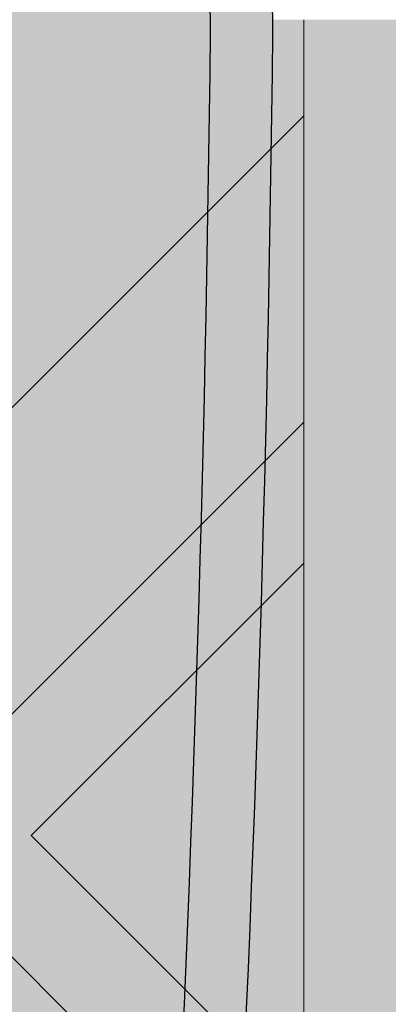
# Model space of a CAD drawing. Units: inches. Extents: x 844 to 2234, y 346 to 1084.
# Tile 11 of 93: x 1126.594 to 1127.536, y 693.702 to 696.22. Entities that reach past the tile are written whole.
import ezdxf

# ---------------------------------------------------------------- set-up
doc = ezdxf.new("R2010")
doc.units = ezdxf.units.IN
doc.header["$MEASUREMENT"] = 0
for name, color, linetype, lineweight in [('A-ANNO-DIMS', 2, 'Continuous', 18), ('furniture', 8, 'Continuous', 18), ('RA-AP-01$0$INT', 35, 'Continuous', 5)]:
    doc.layers.add(name, color=color, linetype=linetype, lineweight=lineweight)
doc.layers.add('RA-AP-01$0$FURN', color=3, linetype='Continuous')
doc.layers.add('RA-AP-01$0$WOOD', color=64, linetype='Continuous')
doc.styles.get("Standard").update_dxf_attribs({"font": 'arial.ttf'})
doc.dimstyles.get("Standard").update_dxf_attribs({"dimtxt": 6, "dimasz": 3, "dimexe": 0.18, "dimexo": 0.0625, "dimgap": 0.09, "dimtad": 0, "dimtih": 1, "dimtoh": 1, "dimdec": 1, "dimzin": 0, "dimdsep": 46, "dimlunit": 3, "dimtxsty": 'Standard', "dimblk": 'ARCHTICK', "dimcen": 0.09, "dimadec": 0, "dimazin": 0, "dimtfac": 1, "dimtdec": 1, "dimtofl": 0, "dimtmove": 0, "dimatfit": 3, "dimfxl": 1, "dimtolj": 1, "dimtzin": 0, "dimarcsym": 0})

# ---------------------------------------------------------------- blocks, each defined once
blk = doc.blocks.new('A$C18D01794')
at = {"layer": 'RA-AP-01$0$INT'}
blk.add_hatch(color=256, dxfattribs=at).paths.add_polyline_path([(4.505206456958071, -6.306712009588038), (5.305206456958072, -6.306712009588038), (5.305206456958072, -7.106712009588038), (5.255206456951893, -7.10671200958804), (5.25520645694868, -6.356712009605972), (4.555206456959269, -6.356712009587461), (4.555206456956052, -7.106712009588038), (4.505206456958073, -7.106712009588038)])
h = blk.add_hatch(color=256, dxfattribs=at)
h.paths.add_polyline_path([(4.585917135068449, -6.356712009588271), (4.555206456959269, -6.35671200958746), (4.555206456959137, -6.387422687716308), (4.874495778835233, -6.706712009592356), (4.90520645695423, -6.676001331474049)])
h.paths.add_polyline_path([(5.255206456948813, -6.387422687716306), (5.255206456948682, -6.356712009605972), (5.224495778822613, -6.356712009605161), (4.905206456953498, -6.676001331474273), (4.935917135072151, -6.706712009592924)])
h.paths.add_polyline_path([(4.935917135072559, -6.706712009592068), (4.905206456953564, -6.737422687710376), (5.255206456951813, -7.087422687708613), (5.255206456951549, -7.026001331471008)])
h.paths.add_polyline_path([(4.555206456956399, -7.026001331471013), (4.555206456956134, -7.087422687708616), (4.905206456953821, -6.737422687710943), (4.874495778835166, -6.70671200959229)])
h = blk.add_hatch(color=256, dxfattribs=at)
h.paths.add_polyline_path([(4.585917135068448, -6.356712009588273), (4.614201406330596, -6.356712009589021), (4.668846067270487, -6.411356670531338), (4.723490728212344, -6.356712009591912), (4.771774999457151, -6.35671200959319), (4.826419660396886, -6.411356670535356), (4.862780050090322, -6.374996280843536), (4.844495778842715, -6.356712009595112), (4.862780050090411, -6.356712009595595), (4.905206456960182, -6.399138416468211), (4.947632863832445, -6.356712009597838), (4.965917135079675, -6.356712009598322), (4.947632863831759, -6.374996280845421), (4.983993253523576, -6.411356670538857), (5.038637914464627, -6.356712009600247), (5.08692218571208, -6.356712009601523), (5.141566846649976, -6.411356670541852), (5.196211507589851, -6.356712009604411), (5.224495778822615, -6.356712009605161), (4.905206456953975, -6.676001331473793)])
h.paths.add_polyline_path([(4.895206456956031, -6.637717060225675), (4.895206456958921, -6.528427738347902), (4.840561796018589, -6.583072399285802)], flags=16)
h.paths.add_polyline_path([(4.915206456955638, -6.637717060226121), (4.969851117895509, -6.583072399288678), (4.915206456957609, -6.528427738348344)], flags=16)
h.paths.add_polyline_path([(4.826419660395175, -6.568930263661755), (4.881064321335613, -6.514285602723745), (4.771774999456703, -6.514285602720857)], flags=16)
h.paths.add_polyline_path([(4.983993253519558, -6.568930263665262), (5.038637914460456, -6.514285602726792), (4.929348592581548, -6.514285602724816)], flags=16)
h.paths.add_polyline_path([(4.881064321336025, -6.494285602723742), (4.826419660397532, -6.439640941782821), (4.771774999457062, -6.494285602720859)], flags=16)
h.paths.add_polyline_path([(4.929348592582019, -6.494285602724817), (5.038637914460982, -6.494285602726792), (4.983993253522945, -6.439640941786327)], flags=16)
h.paths.add_polyline_path([(4.895206456960191, -6.480143467100443), (4.895206456962115, -6.407422687715913), (4.876922185715016, -6.389138416467584), (4.840561796021581, -6.425498806159401)], flags=16)
h.paths.add_polyline_path([(4.915206456958487, -6.480143467100889), (4.969851117899527, -6.425498806162279), (4.933490728206909, -6.389138416468043), (4.9152064569598, -6.40742268771434)], flags=16)
h.paths.add_polyline_path([(4.757632863832376, -6.480143467096812), (4.812277524772842, -6.425498806158772), (4.757632863834348, -6.370854145217844)], flags=16)
h.paths.add_polyline_path([(4.737632863832376, -6.480143467096286), (4.737632863834348, -6.370854145217375), (4.682988202893906, -6.425498806155385)], flags=16)
h.paths.add_polyline_path([(5.05278005008503, -6.480143467103376), (5.052780050087917, -6.370854145224413), (4.998135389146995, -6.425498806162908)], flags=16)
h.paths.add_polyline_path([(5.072780050085024, -6.480143467103744), (5.127424711025931, -6.42549880616527), (5.072780050087916, -6.370854145224832)], flags=16)
h.paths.add_polyline_path([(4.935917135072783, -6.706712009592292), (5.255206456948811, -6.387422687716309), (5.255206456948932, -6.415706958964177), (5.200561796010279, -6.470351619902839), (5.255206456949403, -6.524996280841948), (5.25520645694961, -6.5732805520894), (5.200561796009787, -6.627925213029239), (5.236922185702417, -6.664285602721864), (5.255206456949919, -6.646001331474357), (5.255206456949998, -6.664285602721898), (5.212780050078687, -6.706712009592262), (5.25520645695036, -6.749138416463932), (5.255206456950438, -6.767422687711313), (5.236922185702424, -6.749138416463297), (5.200561796009796, -6.785498806155928), (5.255206456950753, -6.840143467096874), (5.25520645695096, -6.888427738341682), (5.200561796010322, -6.943072399282328), (5.255206456951428, -6.997717060223427), (5.255206456951547, -7.026001331471006)])
h.paths.add_polyline_path([(5.042988202883395, -6.785498806155427), (5.097632863823085, -6.840143467095101), (5.097632863822622, -6.730854145216193)], flags=16)
h.paths.add_polyline_path([(5.028846067259663, -6.771356670531693), (5.083490728198774, -6.716712009592573), (4.974201406321001, -6.716712009593042)], flags=16)
h.paths.add_polyline_path([(5.117632863823087, -6.840143467095186), (5.172277524762331, -6.785498806155926), (5.11763286382262, -6.730854145216225)], flags=16)
h.paths.add_polyline_path([(5.08349072819877, -6.696712009593886), (5.028846067259652, -6.642067348654775), (4.974201406320998, -6.696712009593438)], flags=16)
h.paths.add_polyline_path([(5.131774999446817, -6.854285602718917), (5.186419660386065, -6.799640941779662), (5.241064321325782, -6.854285602719365)], flags=17)
h.paths.add_polyline_path([(5.131774999446228, -6.716712009592374), (5.186419660386065, -6.771356670532194), (5.222780050079488, -6.734996280838764), (5.204495778832781, -6.716712009592063)], flags=16)
h.paths.add_polyline_path([(5.097632863822613, -6.682569873970264), (5.097632863823061, -6.573280552091354), (5.042988202883383, -6.627925213031044)], flags=16)
h.paths.add_polyline_path([(5.131774999446899, -6.874285602718915), (5.241064321325809, -6.874285602719364), (5.186419660386591, -6.928930263658598)], flags=17)
h.paths.add_polyline_path([(5.131774999446226, -6.696712009594078), (5.204495778830767, -6.696712009594374), (5.22278005007868, -6.67842773834687), (5.186419660386049, -6.642067348654249)], flags=16)
h.paths.add_polyline_path([(5.11763286382262, -6.682569873970225), (5.17227752476232, -6.627925213030515), (5.117632863823064, -6.573280552091267)], flags=16)
h.paths.add_polyline_path([(5.186419660386069, -6.613783077405491), (5.241064321325754, -6.559138416465795), (5.131774999446791, -6.559138416466263)], flags=16)
h.paths.add_polyline_path([(5.131774999446872, -6.539138416466263), (5.24106432132578, -6.539138416465794), (5.186419660386554, -6.484493755526573)], flags=16)
h.paths.add_polyline_path([(5.255206456951811, -7.08742268770861), (5.255206456951895, -7.106712009588038), (4.555206456956052, -7.106712009588038), (4.555206456956136, -7.087422687708617), (4.905206456953973, -6.737422687710788)])
h.paths.add_polyline_path([(4.983993253513404, -6.8444937555241), (4.92934859257295, -6.899138416462108), (5.03863791445186, -6.899138416465014)], flags=16)
h.paths.add_polyline_path([(4.969851117889988, -6.83035161990006), (4.915206456952556, -6.775706958960171), (4.915206456949648, -6.884996280837944)], flags=16)
h.paths.add_polyline_path([(4.929348592572535, -6.919138416462105), (4.983993253511019, -6.973783077403037), (5.038637914451496, -6.919138416465012)], flags=16)
h.paths.add_polyline_path([(5.052780050074912, -6.93328055208906), (4.998135389134438, -6.987925213027088), (5.052780050072919, -7.042569873968025)], flags=16)
h.paths.add_polyline_path([(5.07278005007491, -6.933280552089588), (5.072780050072918, -7.042569873968497), (5.127424711013374, -6.987925213030498)], flags=16)
h.paths.add_polyline_path([(4.89520645695295, -6.775706958959721), (4.840561796013067, -6.830351619897157), (4.895206456950961, -6.884996280837494)], flags=16)
h.paths.add_polyline_path([(4.915206456948365, -6.933280552085403), (4.915206456946434, -7.006001331471951), (4.933490728192729, -7.024285602719066), (4.969851117886972, -6.987925213026453)], flags=16)
h.paths.add_polyline_path([(4.881064321327021, -6.899138416461022), (4.82641966038902, -6.84449375552057), (4.771774999448108, -6.899138416459029)], flags=16)
h.paths.add_polyline_path([(4.895206456950073, -6.933280552084951), (4.840561796009022, -6.987925213023558), (4.876922185700835, -7.024285602716997), (4.895206456948749, -7.006001331469487)], flags=16)
h.paths.add_polyline_path([(4.983993253510392, -7.0020673486505), (4.947632863816944, -7.038427738342319), (4.965917135064043, -7.05671200959023), (5.038637914448995, -7.056712009591555)], flags=16)
h.paths.add_polyline_path([(4.881064321326543, -6.91913841646102), (4.771774999447578, -6.919138416459031), (4.826419660385607, -6.973783077399508)], flags=16)
h.paths.add_polyline_path([(4.905206456946447, -7.014285602717636), (4.862780050074785, -7.056712009588352), (4.947632863816685, -7.056712009589775)], flags=16)
h.paths.add_polyline_path([(5.14156684663679, -7.002067348654549), (5.086922185696452, -7.056712009592438), (5.196211507574223, -7.056712009594425)], flags=16)
h.paths.add_polyline_path([(4.8264196603837, -7.002067348646972), (4.771774999442643, -7.056712009585575), (4.8444957788276, -7.056712009587508), (4.862780050075511, -7.038427738340416)], flags=16)
h.paths.add_polyline_path([(4.812277524760289, -6.98792521302292), (4.757632863822258, -6.933280552082447), (4.757632863819352, -7.042569873961408)], flags=16)
h.paths.add_polyline_path([(4.73763286382226, -6.933280552082079), (4.682988202881349, -6.987925213020536), (4.737632863819352, -7.04256987396099)], flags=16)
h.paths.add_polyline_path([(4.723490728195188, -7.056712009584289), (4.668846067257299, -7.002067348643949), (4.614201406317417, -7.056712009581383)], flags=16)
h.paths.add_polyline_path([(4.597632863829262, -6.706712009592262), (4.555206456957951, -6.664285602721896), (4.555206456958029, -6.646001331474357), (4.573490728205535, -6.664285602721864), (4.609851117898167, -6.627925213029238), (4.555206456958338, -6.573280552089402), (4.555206456958546, -6.524996280841952), (4.60985111789767, -6.470351619902839), (4.555206456959015, -6.415706958964177), (4.555206456959138, -6.387422687716309), (4.874495778835167, -6.70671200959229), (4.5552064569564, -7.026001331471015), (4.555206456956523, -6.997717060223433), (4.609851117897629, -6.94307239928233), (4.555206456956988, -6.888427738341681), (4.555206456957198, -6.840143467096881), (4.609851117898153, -6.78549880615593), (4.573490728205528, -6.749138416463297), (4.555206456957507, -6.76742268771132), (4.555206456957585, -6.749138416463933)])
h.paths.add_polyline_path([(4.712780050085332, -6.730854145216195), (4.712780050084863, -6.840143467095105), (4.767424711024555, -6.785498806155427)], flags=16)
h.paths.add_polyline_path([(4.726922185709173, -6.716712009592573), (4.781566846648288, -6.771356670531693), (4.836211507586949, -6.716712009593043)], flags=16)
h.paths.add_polyline_path([(4.692780050085327, -6.730854145216225), (4.638135389145619, -6.785498806155928), (4.692780050084865, -6.840143467095185)], flags=16)
h.paths.add_polyline_path([(4.726922185709182, -6.696712009593886), (4.836211507586949, -6.696712009593436), (4.7815668466483, -6.642067348654773)], flags=16)
h.paths.add_polyline_path([(4.678637914461726, -6.71671200959237), (4.605917135075169, -6.716712009592063), (4.587632863828464, -6.734996280838766), (4.623993253521887, -6.771356670532195)], flags=16)
h.paths.add_polyline_path([(4.712780050085336, -6.68256987397026), (4.767424711024568, -6.627925213031042), (4.71278005008489, -6.573280552091352)], flags=16)
h.paths.add_polyline_path([(4.678637914461726, -6.696712009594076), (4.623993253521899, -6.642067348654247), (4.587632863829271, -6.67842773834687), (4.605917135077185, -6.696712009594376)], flags=16)
h.paths.add_polyline_path([(4.692780050085336, -6.682569873970228), (4.692780050084889, -6.573280552091267), (4.638135389145632, -6.627925213030515)], flags=16)
h.paths.add_polyline_path([(4.623993253521885, -6.799640941779662), (4.678637914461131, -6.854285602718915), (4.56934859258217, -6.854285602719365)], flags=17)
h.paths.add_polyline_path([(4.623993253521901, -6.613783077405509), (4.678637914461158, -6.559138416466263), (4.569348592582195, -6.559138416465795)], flags=16)
h.paths.add_polyline_path([(4.678637914461051, -6.874285602718915), (4.623993253521361, -6.928930263658598), (4.569348592582143, -6.874285602719364)], flags=17)
h.paths.add_polyline_path([(4.678637914461076, -6.539138416466263), (4.623993253521399, -6.484493755526573), (4.569348592582167, -6.539138416465796)], flags=16)
h = blk.add_hatch(color=256, dxfattribs=at)
h.paths.add_polyline_path([(5.028846067259997, -6.642067348655121), (4.974201406321342, -6.696712009593783), (5.083490728199115, -6.69671200959423)])
h.paths.add_polyline_path([(4.974201406321344, -6.716712009593388), (5.028846067260004, -6.771356670532039), (5.083490728199117, -6.716712009592919)])
h.paths.add_polyline_path([(5.042988202883738, -6.785498806155768), (5.097632863823428, -6.840143467095449), (5.097632863822963, -6.73085414521654)])
h.paths.add_polyline_path([(5.117632863822961, -6.730854145216568), (5.117632863823428, -6.840143467095531), (5.172277524762674, -6.785498806156272)])
h.paths.add_polyline_path([(5.131774999446572, -6.716712009592718), (5.186419660386406, -6.77135667053254), (5.222780050079831, -6.734996280839116), (5.204495778833122, -6.716712009592409)])
h.paths.add_polyline_path([(5.236922185702764, -6.749138416463644), (5.200561796010139, -6.785498806156274), (5.255206456949971, -6.840143467096101), (5.255206456950271, -6.76742268771115)])
h.paths.add_polyline_path([(5.186419660386412, -6.799640941780006), (5.131774999447164, -6.854285602719262), (5.241064321326123, -6.854285602719711)])
h.paths.add_polyline_path([(5.131774999447238, -6.874285602719261), (5.186419660386934, -6.928930263658944), (5.241064321326153, -6.874285602719709)])
h.paths.add_polyline_path([(5.200561796010663, -6.943072399282675), (5.255206456949324, -6.997717060221329), (5.255206456949777, -6.888427738343558)])
h.paths.add_polyline_path([(5.21278005007903, -6.706712009592607), (5.255206456950223, -6.749138416463798), (5.255206456950696, -6.664285602721891)])
h.paths.add_polyline_path([(5.13177499944657, -6.696712009594424), (5.204495778831106, -6.696712009594723), (5.222780050079024, -6.678427738347219), (5.186419660386397, -6.642067348654592)])
h.paths.add_polyline_path([(5.117632863823405, -6.573280552091611), (5.117632863822955, -6.682569873970578), (5.172277524762665, -6.627925213030859)])
h.paths.add_polyline_path([(5.042988202883727, -6.627925213031387), (5.097632863822957, -6.682569873970603), (5.097632863823407, -6.573280552091697)])
h.paths.add_polyline_path([(5.131774999447135, -6.559138416466609), (5.186419660386394, -6.613783077405857), (5.241064321326097, -6.559138416466144)])
h.paths.add_polyline_path([(5.200561796010128, -6.627925213029584), (5.236922185702758, -6.664285602722211), (5.255206456950264, -6.646001331474705), (5.255206456949948, -6.573280552089752)])
h.paths.add_polyline_path([(5.186419660386895, -6.484493755526919), (5.131774999447213, -6.539138416466609), (5.241064321326127, -6.539138416466142)])
h.paths.add_polyline_path([(5.200561796010624, -6.470351619903183), (5.255206456949745, -6.524996280842298), (5.255206456949276, -6.415706958964523)])
for p, q in [((5.255206456951895, -7.106712009588038), (5.255206456948681, -6.356712009605972)), ((4.935917135072783, -6.706712009592292), (5.255206456951548, -7.026001331471007)), ((4.905206456953975, -6.737422687710788), (5.255206456951811, -7.087422687708611)), ((5.241064321325809, -6.874285602719364), (5.186419660386589, -6.928930263658598)), ((5.255206456949429, -6.888427738343214), (5.200561796010322, -6.943072399282328)), ((5.255206456949433, -6.888427738343212), (5.255206456948982, -6.997717060220983)), ((5.255206456948982, -6.997717060220983), (5.200561796010322, -6.943072399282328))]:
    blk.add_line(p, q, dxfattribs=at)
blk = doc.blocks.new('A$C32926AE1')
at = {"layer": 'RA-AP-01$0$WOOD'}
h = blk.add_hatch(color=256, dxfattribs=at)
h.dxf.hatch_style = 1
h.paths.add_polyline_path([(5.157430609644524, 4.573483066760929, -0.1009492694046607), (5.155401577623758, 4.593365984175333, -0.1842662638101597), (5.172249623284174, 4.638795604568598, 0.2056608120311276), (5.179560981299304, 4.661316324430096, 0.3614336704623542), (5.134352340494423, 4.706524965234944, 0.2056608120311297), (5.111831620632933, 4.699213607219793, -0.1842662638101113), (5.066402000239693, 4.682365561559342, -0.1055311479399994), (5.045656153913092, 4.68467289944697, 0.1567636581983829), (4.763886414745334, 4.684672899446966, -0.1055311479399895), (4.743140568418733, 4.68236556155934, -0.1842662638100833), (4.6977109480255, 4.69921360721979, 0.2056608120302612), (4.675190228164109, 4.706524965234949, 0.3614336704708441), (4.629981587358889, 4.66131632442871, 0.2056608120245944), (4.637292945374126, 4.638795604567974, -0.1842662638101024), (4.654140991034615, 4.59336598417475, -0.1009492694055169), (4.652111959013835, 4.573483066760181, 0.021410119221476), (4.629748025606143, 4.156712009541676, 0.0214101192214795), (4.652111959013809, 3.739940952323101, -0.1009492694059586), (4.654140991034615, 3.720058034908448, -0.1842662638100975), (4.637292945374126, 3.674628414515226, 0.2056608120245705), (4.629981587358889, 3.652107694654492, 0.3614336704708879), (4.675190228164113, 3.606899053848249, 0.2056608120302384), (4.697710948025501, 3.614210411863408, -0.1842662638100995), (4.743140568418738, 3.63105845752386, -0.1055311479402541), (4.763886414745388, 3.628751119636215, 0.1567636581983776), (5.045656153913137, 3.628751119636244, -0.1055311479397538), (5.066402000239692, 3.631058457523857, -0.1842662638101067), (5.111831620632931, 3.614210411863407, 0.2056608120310924), (5.134352340494417, 3.606899053848256, 0.3614336704624001), (5.179560981299307, 3.652107694653103, 0.2056608120311314), (5.172249623284175, 3.6746284145146, -0.1842662638101402), (5.155401577623758, 3.72005803490786, -0.1009492694051366), (5.15743060964455, 3.739940952322354, 0.0214101192215073), (5.179794543052287, 4.156712009541468, 0.0214101192215252)])
h.paths.add_polyline_path([(4.639748609479751, 4.156712009541513, 0.0213537860821624), (4.661970494867118, 3.741887061152232, -0.094075836301374), (4.664143710413708, 3.7196126951003, -0.1824818158568985), (4.644813765429836, 3.668037719127816, 0.2056608120245319), (4.639939526753007, 3.653023905887301, 0.3614336704710246), (4.676106439397173, 3.616856993242342, 0.2056608120302234), (4.691120252638095, 3.621731231919122, -0.1824818158602558), (4.742695228611606, 3.641061176902986, -0.1029891339458722), (4.766991894714349, 3.638256818950944, 0.156709409989566), (5.042550673941472, 3.638256818950105, -0.102989133958497), (5.066847340047078, 3.641061176902949, -0.1824818158594995), (5.118422316020358, 3.621731231919103, 0.2056608120311416), (5.133436129261316, 3.616856993242346, 0.3614336704621468), (5.169603041905217, 3.653023905886178, 0.2056608120310986), (5.164728803228477, 3.668037719127177, -0.1824818158565612), (5.145398858244737, 3.719612695099578, -0.0940758363009313), (5.147572073791232, 3.741887061151398, 0.0213537860822023), (5.169793959178681, 4.156712009541451, 0.0213537860822226), (5.147572073791203, 4.571536957931898, -0.0940758363005034), (5.145398858244737, 4.59381132398362, -0.1824818158565587), (5.164728803228476, 4.645386299956021, 0.2056608120311045), (5.169603041905216, 4.66040011319702, 0.3614336704621845), (5.133436129261313, 4.696567025840856, 0.2056608120310773), (5.118422316020359, 4.691692787164098, -0.182481815859508), (5.066847340047078, 4.67236284218025, -0.1029891339584606), (5.04255067394148, 4.675167200133092, 0.156709409989566), (4.766991894714357, 4.675167200132257, -0.1029891339458842), (4.742695228611611, 4.672362842180213, -0.1824818158602725), (4.691120252638095, 4.691692787164077, 0.2056608120302152), (4.676106439397174, 4.696567025840858, 0.3614336704710363), (4.639939526753005, 4.660400113195899, 0.2056608120245495), (4.644813765429837, 4.645386299955384, -0.1824818158568934), (4.664143710413708, 4.593811323982902, -0.0940758363009187), (4.661970494867149, 4.571536957931074, 0.021353786082177)], flags=16)
h.paths.add_polyline_path([(5.129794543052235, 4.432167055276933, -0.0141661062790638), (5.130152669293814, 4.156927903047693, -0.0141661062790647), (5.129794543052234, 3.881688750818433, -0.0785247771143638), (5.10979738006795, 3.755143611847103, 0.0945969212073497), (5.105408519571111, 3.717898134952927, 0.1043170707844957), (5.116074640131521, 3.670385395016088, 0.1043170707864965), (5.068561900193738, 3.681051515576561, 0.09459692119553), (5.031316423304057, 3.676662655080835, -0.1580239521427272), (4.778226145355827, 3.676662655080367, 0.0945969211986668), (4.740980668464973, 3.681051515576592, 0.1043170707882822), (4.693467928526415, 3.670385395015844, 0.1043170707867916), (4.704134049087309, 3.717898134953662, 0.0945969211972894), (4.69974518859162, 3.755143611844042, -0.0785247771163196), (4.679748025606343, 3.881688750818406, -0.0141661062790663), (4.679389899364763, 4.156927903047693, -0.0141661062790672), (4.679748025606343, 4.432167055276998, -0.0785247771163064), (4.699745188591625, 4.55871219425134, 0.094596921197333), (4.704134049087308, 4.595957671141738, 0.1043170707867205), (4.693467928526416, 4.643470411079523, 0.1043170707882628), (4.740980668464965, 4.632804290518776, 0.0945969211988114), (4.778226145355874, 4.637193151015016, -0.158023952142669), (5.031316423304015, 4.637193151014546, 0.0945969211956361), (5.068561900193736, 4.632804290518806, 0.1043170707864979), (5.11607464013152, 4.643470411079278, 0.1043170707844617), (5.105408519571112, 4.595957671142455, 0.0945969212074597), (5.109797380067959, 4.558712194248236, -0.0785247771143467)], flags=0)
h.paths.add_polyline_path([(5.119794532311105, 4.432259799204851, -0.0142000800617244), (5.120156169157484, 4.156927903047701, -0.0142000800617277), (5.119794532311105, 3.881596006890482, -0.0784894509520253), (5.100273383573699, 3.758192358677797, 0.0940138827242913), (5.095413455884425, 3.717477693979438, 0.0606271852308753), (5.099615656341024, 3.686844378806616, 0.0606271852322524), (5.068982341167493, 3.691046579263239, 0.0940138827010453), (5.028267676478798, 3.686186651576848, -0.1580706864508061), (4.781274892180912, 3.686186651576435, 0.0940138827026903), (4.740560227491556, 3.691046579263279, 0.0606271852339895), (4.709926912317155, 3.686844378806508, 0.0606271852329405), (4.714129112773991, 3.717477693980356, 0.094013882701304), (4.709269185087677, 3.758192358669163, -0.0784894509577193), (4.689748036347473, 3.881596006890469, -0.014200080061729), (4.689386399501094, 4.156927903047709, -0.0142000800617217), (4.689748036347473, 4.432259799204808, -0.078489450957724), (4.709269185087651, 4.555663447426125, 0.0940138827014585), (4.714129112773992, 4.596378112114996, 0.0606271852329731), (4.709926912317154, 4.62701142728886, 0.0606271852340196), (4.74056022749157, 4.622809226832087, 0.0940138827024997), (4.781274892180847, 4.627669154518912, -0.1580706864508359), (5.028267676478777, 4.627669154518526, 0.0940138827010946), (5.068982341167492, 4.622809226832129, 0.060627185232254), (5.099615656341024, 4.627011427288751, 0.0606271852308727), (5.095413455884425, 4.59637811211593, 0.0940138827241088), (5.100273383573675, 4.555663447417647, -0.0784894509520978)], flags=0)
h.paths.add_polyline_path([(5.06978912287499, 4.430218106756144, -0.014241683694547), (5.070173729147532, 4.156927903047672, -0.0142416836945458), (5.06978912287499, 3.883637699339223, -0.0800609523125196), (5.052662118612511, 3.773463122773442, 0.0526421978001116), (5.04590916754064, 3.740550867606997, 0.0526421977992423), (5.012996912374707, 3.73379791653534, -0.1583028414718258), (4.796545656286308, 3.73379791653451, 0.0526421978034211), (4.763633401117837, 3.740550867607021, 0.0526421978018622), (4.756880450045755, 3.773463122774558, -0.0800609523117106), (4.739753445783639, 3.883637699339268, -0.0142416836945435), (4.739368839511098, 4.156927903047671, -0.0142416836945477), (4.739753445783639, 4.430218106756155, -0.0800609523116345), (4.75688045004574, 4.540392683320762, 0.052642197801941), (4.763633401117837, 4.573304938488346, 0.0526421978035071), (4.796545656286361, 4.580057889560873, -0.1583028414717561), (5.012996912374669, 4.580057889560039, 0.0526421977993048), (5.04590916754064, 4.57330493848837, 0.0526421978002057), (5.052662118612529, 4.540392683321868, -0.080060952312477)], flags=0)
h.paths.add_polyline_path([(5.049789715110557, 4.43038092723357, -0.0143097550741839), (5.05018085590259, 4.156927903047715, -0.0143097550741854), (5.049789715110558, 3.883474878861827, -0.0800685599149176), (5.03362098255317, 3.779581877367999, 0.0306258898956367), (5.028241146483733, 3.758218888663947, 0.0306258898977031), (5.006878157778253, 3.75283905259408, -0.1583983521624096), (4.802664410878162, 3.752839052594731, 0.0306258898946014), (4.781301422174808, 3.758218888663924, 0.0306258898967912), (4.775921586105202, 3.779581877368794, -0.080068559914251), (4.759752853548071, 3.883474878861786, -0.0143097550741854), (4.759361712756037, 4.156927903047671, -0.0143097550741854), (4.759752853548071, 4.430380927233557, -0.0800685599142479), (4.775921586105193, 4.534273928726546, 0.0306258898968306), (4.781301422174808, 4.555636917431444, 0.0306258898945754), (4.802664410878143, 4.561016753500631, -0.1583983521624168), (5.006878157778244, 4.561016753501291, 0.0306258898977177), (5.028241146483733, 4.555636917431421, 0.0306258898958182), (5.03362098255321, 4.534273928727244, -0.080068559914796)], flags=0)
h.paths.add_polyline_path([(4.999766070382627, 4.428171244713864, -0.0143443147609634), (5.000198441819402, 4.156927903047689, -0.0143443147609612), (4.999766070382627, 3.885684561381556, -0.0784641635803329), (4.987356730658798, 3.799103304488872, -0.1506053783831347), (4.822185837999821, 3.79910330448882, -0.0784641635803318), (4.809776498276007, 3.885684561381509, -0.014344314760963), (4.809344126839227, 4.156927903047677, -0.0143443147609645), (4.809776498276007, 4.428171244713873, -0.0784641635803192), (4.822185837999822, 4.514752501606549, -0.1506053783831338), (4.987356730658798, 4.514752501606494, -0.078464163580285)], flags=0)
h.paths.add_polyline_path([(4.979755254238824, 4.42764379880488, -0.0143772539198268), (4.980205517789977, 4.156927903047693, -0.0143772539198275), (4.979755254238824, 3.886212007290489, -0.0689242507424422), (4.971183264704897, 3.815276770442801, -0.1296645318904179), (4.838359303953726, 3.815276770442746, -0.0689242507424186), (4.829787314419809, 3.886212007290419, -0.0143772539198292), (4.829337050868653, 4.156927903047653, -0.0143772539198325), (4.829787314419809, 4.427643798804946, -0.0689242507424211), (4.838359303953725, 4.498579035652621, -0.1296645318904187), (4.971183264704897, 4.498579035652565, -0.0689242507424401)], flags=0)
h = blk.add_hatch(color=256, dxfattribs=at)
h.dxf.hatch_style = 1
h.paths.add_polyline_path([(5.145398858244737, 4.59381132398362, -0.1824818158565616), (5.164728803228476, 4.645386299956021, 0.2056608120311045), (5.169603041905216, 4.66040011319702, 0.3614336704621845), (5.133436129261313, 4.696567025840856, 0.2056608120310773), (5.118422316020359, 4.691692787164098, -0.182481815859508), (5.066847340047078, 4.67236284218025, -0.1029891339584606), (5.04255067394148, 4.675167200133092, 0.156709409989566), (4.766991894714357, 4.675167200132257, -0.1029891339458842), (4.742695228611611, 4.672362842180213, -0.1824818158602725), (4.691120252638095, 4.691692787164077, 0.2056608120302152), (4.676106439397174, 4.696567025840858, 0.3614336704710363), (4.639939526753005, 4.660400113195899, 0.2056608120245495), (4.644813765429837, 4.645386299955384, -0.1824818158568934), (4.664143710413708, 4.593811323982902, -0.0940758363009187), (4.661970494867149, 4.571536957931074, 0.0213537860821772), (4.639748609479751, 4.156712009541507, 0.0213537860821625), (4.661970494867119, 3.741887061152226, -0.0940758363013071), (4.664143710413708, 3.719612695100309, -0.1824818158569294), (4.644813765429836, 3.668037719127816, 0.2056608120245319), (4.639939526753007, 3.653023905887301, 0.3614336704710246), (4.676106439397173, 3.616856993242342, 0.2056608120302234), (4.691120252638095, 3.621731231919122, -0.1824818158602558), (4.742695228611606, 3.641061176902986, -0.1029891339458722), (4.766991894714349, 3.638256818950944, 0.156709409989566), (5.042550673941472, 3.638256818950105, -0.102989133958497), (5.066847340047078, 3.641061176902949, -0.1824818158594995), (5.118422316020358, 3.621731231919103, 0.2056608120311416), (5.133436129261316, 3.616856993242346, 0.3614336704621468), (5.169603041905217, 3.653023905886178, 0.2056608120310986), (5.164728803228477, 3.668037719127177, -0.1824818158565612), (5.145398858244737, 3.719612695099578, -0.0940758363009313), (5.147572073791232, 3.741887061151398, 0.0213537860822023), (5.169793959178681, 4.156712009541451, 0.0213537860822226), (5.147572073791203, 4.571536957931898, -0.0940758363004996)])
h.paths.add_polyline_path([(5.109797380067958, 4.55871219424824, -0.0785247771143472), (5.129794543052234, 4.432167055276936, -0.0141661062790644), (5.130152669293814, 4.156927903047685, -0.014166106279066), (5.129794543052234, 3.881688750818401, -0.0785247771143517), (5.109797380067946, 3.755143611847092, 0.0945969212073132), (5.105408519571111, 3.717898134952929, 0.1043170707844995), (5.116074640131521, 3.670385395016088, 0.1043170707864965), (5.068561900193738, 3.681051515576561, 0.09459692119553), (5.031316423304057, 3.676662655080835, -0.1580239521427272), (4.778226145355827, 3.676662655080367, 0.0945969211986668), (4.740980668464973, 3.681051515576592, 0.1043170707882822), (4.693467928526415, 3.670385395015844, 0.1043170707867916), (4.704134049087309, 3.717898134953662, 0.0945969211972894), (4.69974518859162, 3.755143611844042, -0.0785247771163196), (4.679748025606343, 3.881688750818406, -0.0141661062790663), (4.679389899364763, 4.156927903047693, -0.0141661062790672), (4.679748025606343, 4.432167055276998, -0.0785247771163064), (4.699745188591625, 4.55871219425134, 0.094596921197333), (4.704134049087308, 4.595957671141738, 0.1043170707867205), (4.693467928526416, 4.643470411079523, 0.1043170707882628), (4.740980668464965, 4.632804290518776, 0.0945969211988114), (4.778226145355874, 4.637193151015016, -0.158023952142669), (5.031316423304015, 4.637193151014546, 0.0945969211956361), (5.068561900193736, 4.632804290518806, 0.1043170707864979), (5.11607464013152, 4.643470411079278, 0.1043170707844617), (5.105408519571112, 4.595957671142455, 0.0945969212074504)], flags=16)
h.paths.add_polyline_path([(5.100273383573655, 4.55566344741771, -0.0784894509521388), (5.119794532311105, 4.432259799204852, -0.0142000800617252), (5.120156169157484, 4.156927903047686, -0.014200080061726), (5.119794532311105, 3.881596006890502, -0.0784894509520446), (5.100273383573696, 3.758192358677786, 0.0940138827242721), (5.095413455884425, 3.717477693979436, 0.0606271852308692), (5.099615656341024, 3.686844378806616, 0.0606271852322522), (5.068982341167493, 3.691046579263239, 0.0940138827010453), (5.028267676478798, 3.686186651576848, -0.1580706864508061), (4.781274892180912, 3.686186651576435, 0.0940138827026903), (4.740560227491556, 3.691046579263279, 0.0606271852339895), (4.709926912317155, 3.686844378806508, 0.0606271852329405), (4.714129112773991, 3.717477693980356, 0.094013882701304), (4.709269185087677, 3.758192358669163, -0.0784894509577193), (4.689748036347473, 3.881596006890469, -0.014200080061729), (4.689386399501094, 4.156927903047709, -0.0142000800617217), (4.689748036347473, 4.432259799204808, -0.078489450957724), (4.709269185087651, 4.555663447426125, 0.0940138827014585), (4.714129112773992, 4.596378112114996, 0.0606271852329731), (4.709926912317154, 4.62701142728886, 0.0606271852340196), (4.74056022749157, 4.622809226832087, 0.0940138827024997), (4.781274892180847, 4.627669154518912, -0.1580706864508359), (5.028267676478777, 4.627669154518526, 0.0940138827010946), (5.068982341167492, 4.622809226832129, 0.060627185232254), (5.099615656341024, 4.627011427288751, 0.0606271852308727), (5.095413455884425, 4.59637811211593, 0.094013882723957)], flags=0)
h.paths.add_polyline_path([(5.04590916754064, 4.57330493848837, 0.0526421978002057), (5.052662118612529, 4.540392683321868, -0.0800609523124783), (5.06978912287499, 4.430218106756142, -0.0142416836945469), (5.070173729147532, 4.156927903047672, -0.0142416836945458), (5.06978912287499, 3.883637699339223, -0.0800609523125196), (5.052662118612511, 3.773463122773442, 0.0526421978001116), (5.04590916754064, 3.740550867606997, 0.0526421977992423), (5.012996912374707, 3.73379791653534, -0.1583028414718258), (4.796545656286308, 3.73379791653451, 0.0526421978034211), (4.763633401117837, 3.740550867607021, 0.0526421978018622), (4.756880450045755, 3.773463122774558, -0.0800609523117106), (4.739753445783639, 3.883637699339268, -0.0142416836945435), (4.739368839511098, 4.156927903047671, -0.0142416836945477), (4.739753445783639, 4.430218106756155, -0.0800609523116345), (4.75688045004574, 4.540392683320762, 0.052642197801941), (4.763633401117837, 4.573304938488346, 0.0526421978035071), (4.796545656286361, 4.580057889560873, -0.1583028414717561), (5.012996912374669, 4.580057889560039, 0.0526421977993048)], flags=0)
h.paths.add_polyline_path([(5.028241146483733, 4.555636917431422, 0.0306258898956949), (5.033620982553182, 4.534273928727329, -0.0800685599148649), (5.049789715110557, 4.430380927233569, -0.0143097550741839), (5.05018085590259, 4.156927903047715, -0.0143097550741854), (5.049789715110558, 3.883474878861827, -0.0800685599149176), (5.03362098255317, 3.779581877367999, 0.0306258898956367), (5.028241146483733, 3.758218888663947, 0.0306258898977031), (5.006878157778253, 3.75283905259408, -0.1583983521624096), (4.802664410878162, 3.752839052594731, 0.0306258898946014), (4.781301422174808, 3.758218888663924, 0.0306258898967912), (4.775921586105202, 3.779581877368794, -0.080068559914251), (4.759752853548071, 3.883474878861786, -0.0143097550741854), (4.759361712756037, 4.156927903047671, -0.0143097550741854), (4.759752853548071, 4.430380927233557, -0.0800685599142479), (4.775921586105193, 4.534273928726546, 0.0306258898968306), (4.781301422174808, 4.555636917431444, 0.0306258898945754), (4.802664410878143, 4.561016753500631, -0.1583983521624168), (5.006878157778244, 4.561016753501291, 0.0306258898977174)], flags=0)
h.paths.add_polyline_path([(4.987356730658798, 4.514752501606494, -0.0784641635803018), (4.999766070382627, 4.428171244713845, -0.0143443147609637), (5.000198441819402, 4.156927903047665, -0.0143443147609622), (4.999766070382628, 3.885684561381514, -0.0784641635802952), (4.987356730658797, 3.799103304488872, -0.1506053783831338), (4.822185837999821, 3.799103304488819, -0.0784641635803342), (4.809776498276007, 3.885684561381512, -0.0143443147609628), (4.809344126839227, 4.156927903047676, -0.0143443147609646), (4.809776498276007, 4.428171244713873, -0.0784641635803192), (4.822185837999822, 4.514752501606549, -0.1506053783831338)], flags=0)
h.paths.add_polyline_path([(4.971183264704897, 4.498579035652566, -0.0689242507424384), (4.979755254238824, 4.427643798804883, -0.0143772539198276), (4.980205517789977, 4.15692790304768, -0.0143772539198258), (4.979755254238823, 3.88621200729051, -0.0689242507424628), (4.971183264704897, 3.815276770442801, -0.129664531890417), (4.838359303953726, 3.815276770442746, -0.0689242507424186), (4.829787314419809, 3.886212007290419, -0.0143772539198292), (4.829337050868653, 4.156927903047653, -0.0143772539198325), (4.829787314419809, 4.427643798804946, -0.0689242507424211), (4.838359303953725, 4.498579035652621, -0.1296645318904187)], flags=0)
for centre, radius, start, end in [((0.304323780376417, 4.104079819130551), 4.875754844654793, 0.6185013483537143, 5.524589681839913), ((0.304323780376417, 4.104079819130551), 4.865754844654794, 0.6185013483537143, 5.512956158076888), ((0.304323780376417, 4.209344199952462), 4.865754844654794, 354.4870438419264, 359.3814986516463), ((0.304323780376417, 4.209344199952462), 4.875754844654793, 354.4754103181601, 359.3814986516463)]:
    blk.add_arc(centre, radius, start, end, dxfattribs=at)
blk = doc.blocks.new('A$C5D2F253E')
at = {"layer": 'RA-AP-01$0$FURN', "xscale": -0.7999999999883585, "yscale": 0.7999999999883585, "zscale": 0.8, "rotation": 90}
blk.add_blockref('A$C18D01794', (-5.687757199772477, 4.75791982714071), dxfattribs=at)
at = {"layer": 'RA-AP-01$0$WOOD', "rotation": 270}
blk.add_blockref('A$C32926AE1', (-4.161339601644158, 5.73852594588169), dxfattribs=at)
blk = doc.blocks.new('_ArchTick')
at = {"color": 0, "linetype": 'ByBlock', "const_width": 0.15}
blk.add_lwpolyline([(-0.5, -0.5), (0.5, 0.5)], dxfattribs=at)
blk = doc.blocks.new('*D144')
at = {"layer": 'A-ANNO-DIMS', "color": 0, "lineweight": -2, "transparency": 16777216}
for p, q in [((1096.615948, 439.3732739999999), (1096.615948, 1074.743301)), ((1143.115948, 492.373274), (1143.115948, 1074.743301)), ((1096.615948, 1074.563301), (1102.481950728513, 1074.563301)), ((1143.115948, 1074.563301), (1137.249945271487, 1074.563301))]:
    blk.add_line(p, q, dxfattribs=at)
at = {"layer": 'Defpoints', "color": 0, "transparency": 16777216}
for p in [(1143.115948, 1074.563301), (1143.115948, 492.3107739999999), (1096.615948, 439.3107739999999)]:
    blk.add_point(p, dxfattribs=at)
at = {"layer": 'A-ANNO-DIMS', "color": 0, "lineweight": -2, "transparency": 16777216, "xscale": 3, "yscale": 3, "zscale": 3, "rotation": 180}
blk.add_blockref('_ArchTick', (1096.615948, 1074.563301), dxfattribs=at)
at = {"layer": 'A-ANNO-DIMS', "color": 0, "lineweight": -2, "transparency": 16777216, "xscale": 3, "yscale": 3, "zscale": 3}
blk.add_blockref('_ArchTick', (1143.115948, 1074.563301), dxfattribs=at)
at = {"layer": 'A-ANNO-DIMS', "color": 0, "transparency": 16777216, "insert": (1119.865948, 1074.563301), "char_height": 6, "attachment_point": 5}
blk.add_mtext('\\A1;3\'-10 1/2"', dxfattribs=at)

msp = doc.modelspace()

# ---------------------------------------------------------------- block references
at = {"layer": 'furniture', "xscale": 15.94108302203742, "yscale": 15.94108302203742, "zscale": 15.94108302203742, "rotation": 90}
msp.add_blockref('A$C5D2F253E', (1136.147844094663, 696.2584716700112), dxfattribs=at)

# ---------------------------------------------------------------- dimensions: what is measured, and where the dimension line sits
at = {"layer": 'A-ANNO-DIMS'}
dim = msp.add_linear_dim(base=(1143.115948, 1074.563301), p1=(1096.615948, 439.3107739999999), p2=(1143.115948, 492.3107739999999), dimstyle='Standard', override={"dimdec": 1, "dimlfac": 1, "dimrnd": 0, "dimzin": 1, "dimdsep": 46, "dimlunit": 4, "dimfrac": 2}, dxfattribs=at)
dim.commit()
dim.dimension.update_dxf_attribs({"geometry": '*D144', "text_midpoint": (1119.865948, 1074.563301)})

doc.saveas('drawing.dxf')
